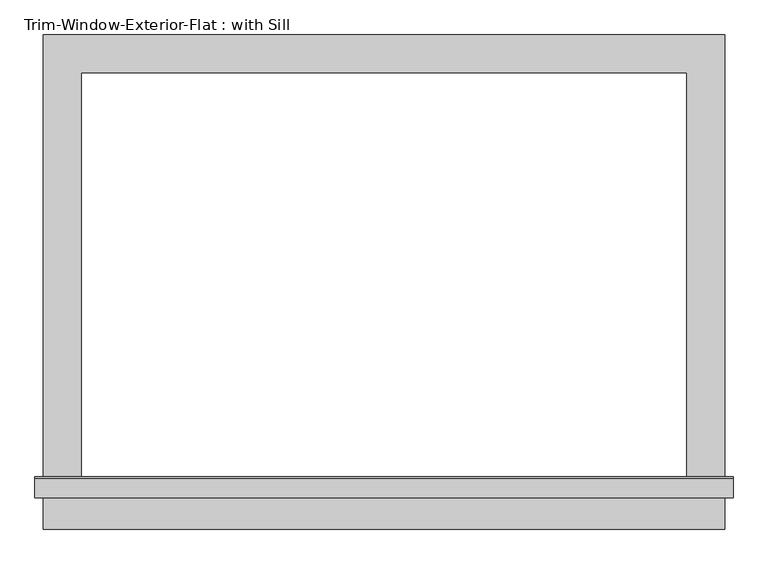
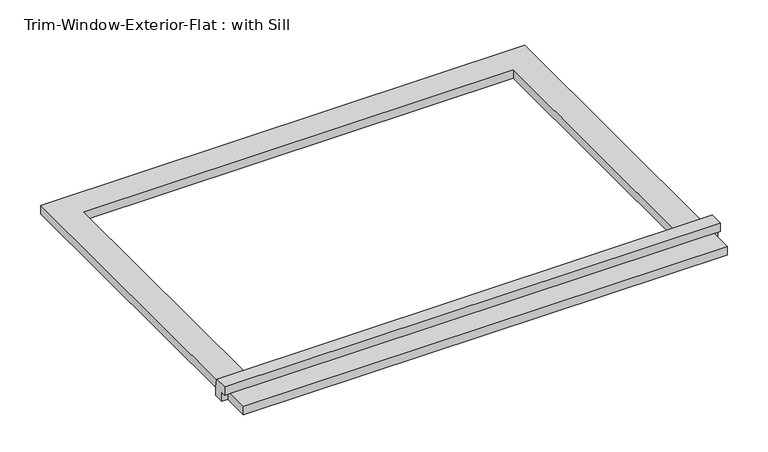
"""IFC4 building model written with IfcOpenShell, lengths in millimetres: proxy geometry, Trim-Window-Exterior-Flat : with Sill."""

from ifc_helpers import new_model, si_unit, frame, origin, origin_with_axes, place, context, project, spatial, polyline, outline, extrude, source, transform, mapped, element, save


def trim_window_exterior_flat_with_sill_40e754a6(model_context):
    return source(origin(), model_context, "Body", "SweptSolid", [
        extrude(outline(polyline([(514.35, -631.7823709), (514.35, -688.9323709), (-514.35, -688.9323709), (-514.35, -631.7823709), (514.35, -631.7823709)])), origin_with_axes(), (0.0, 0.0, 1.0), 19.05),
        extrude(outline(polyline([(-641.35, 38.1), (-612.0580645, 38.1), (-609.6, 19.05), (-609.6, 0.0), (-631.7823709, 0.0), (-631.7823709, 19.05), (-641.35, 19.05), (-641.35, 38.1)])), frame((-527.05, 0.0, 0.0), z_axis=(1.0, 0.0, 0.0), x_axis=(0.0, 1.0, 0.0)), (0.0, 0.0, 1.0), 1054.1),
        extrude(outline(polyline([(-514.35, 57.15), (514.35, 57.15), (514.35, -609.6), (457.2, -609.6), (457.2, 0.0), (-457.2, 0.0), (-457.2, -609.6), (-514.35, -609.6), (-514.35, 57.15)])), origin_with_axes(), (0.0, 0.0, 1.0), 19.05),
    ])


if __name__ == "__main__":
    model = new_model("IFC4")
    model_context = context("Model", 3, world=origin())
    ifc_project = project(units=[si_unit("LENGTHUNIT", "METRE", prefix="MILLI")], contexts=[model_context])
    site = spatial("IfcSite", under=ifc_project)
    building = spatial("IfcBuilding", under=site)
    placement = place(None, origin())
    trim_window_exterior_flat_with_sill_shape = trim_window_exterior_flat_with_sill_40e754a6(model_context)
    element("IfcBuildingElementProxy", 1, Name="Trim-Window-Exterior-Flat : with Sill", ObjectType="Trim-Window-Exterior-Flat : with Sill", at=placement, inside=building, context=model_context, shape_type="MappedRepresentation", body=[
        mapped(trim_window_exterior_flat_with_sill_shape, transform((0.0, 0.0, 0.0), x_axis=(1.0, 0.0, 0.0), y_axis=(0.0, 1.0, 0.0), z_axis=(0.0, 0.0, 1.0))),
    ])
    save(model, "model.ifc")

# Revit data of these elements
# Type "Trim-Window-Exterior-Flat : with Sill"
#   Trim Width = 2.25"
#   Trim Thickness_Picture Frame = 1.25"
#   Trim Thickness_with Sill = 0.75"
#   Sill Thickness = 1.25"
#   Opening Width [instance default] = 24"
#   Opening Height [instance default] = 36"
#   Default Elevation = 48"
#   Sill = yes
#   Picture Frame = no
#   Trim Material [instance default] = none
# Element 1 (IfcBuildingElementProxy, "Trim-Window-Exterior-Flat : with Sill")
#   Opening Width = 36"
#   Opening Height = 24"
#   Trim Material = Clad - White
#   Materials on its faces: "Clad - White"
# Materials
#   "Clad - White": class "Wood", colour RGB 242 242 238, transparency 0, Cost = 0
